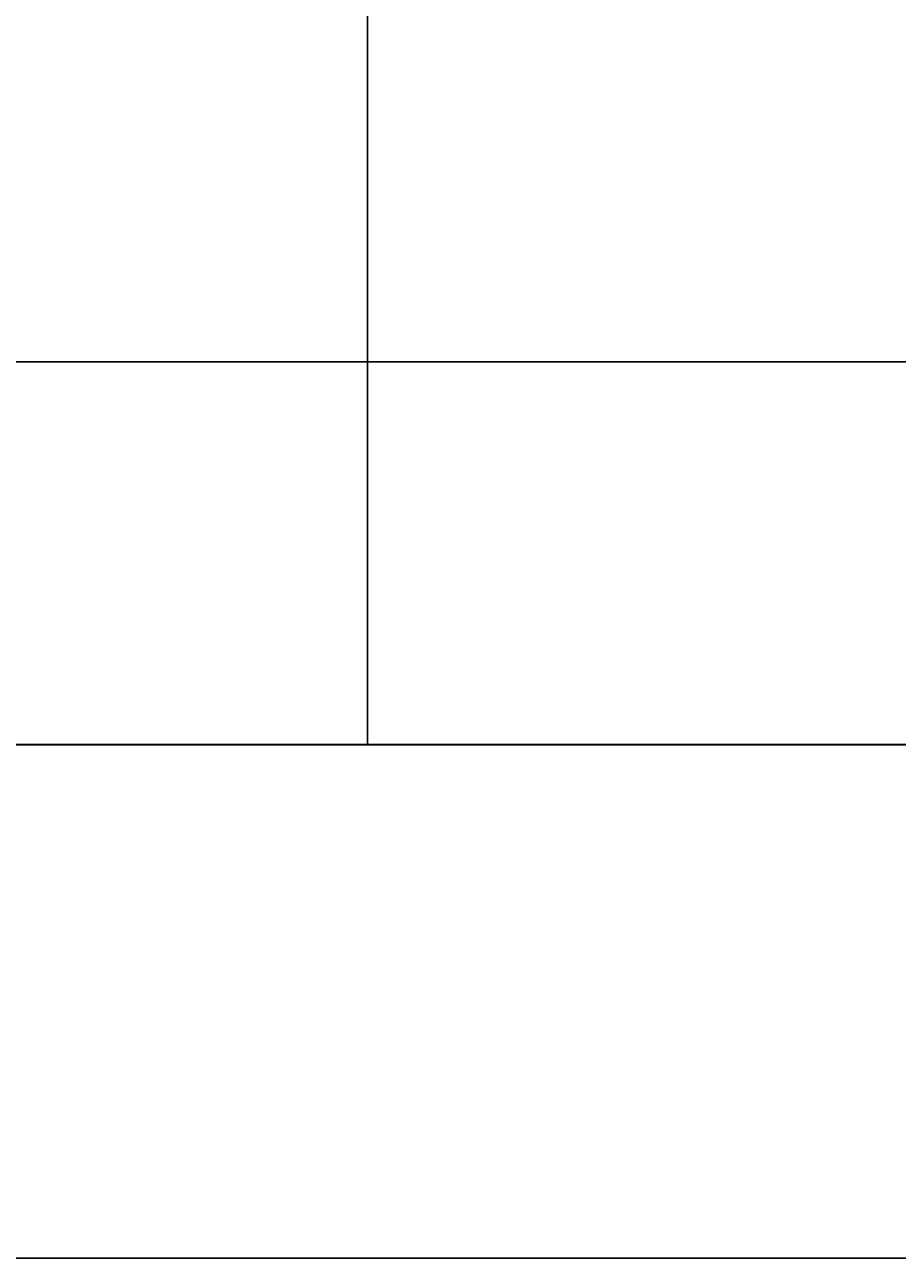
# Model space of a CAD drawing. Units: inches. Extents: x -26 to 776, y -22 to 650.
# Tile 2 of 62: x 36 to 98, y -22 to 67. Entities that reach past the tile are written whole.
import ezdxf

# ---------------------------------------------------------------- set-up
doc = ezdxf.new("R2010")
doc.units = ezdxf.units.IN
doc.header["$MEASUREMENT"] = 0
for name, color, linetype, lineweight in [('A-ANNO-DIMS', 2, 'Continuous', 18), ('A-DOOR', 3, 'Continuous', 25), ('C-TOPO', 7, 'Continuous', 35)]:
    doc.layers.add(name, color=color, linetype=linetype, lineweight=lineweight)
doc.styles.get("Standard").update_dxf_attribs({"font": 'arial.ttf'})
doc.dimstyles.get("Standard").update_dxf_attribs({"dimtxt": 0.5625, "dimasz": 0.18, "dimexe": 0.18, "dimexo": 0.0625, "dimgap": 0.09, "dimtad": 0, "dimtih": 1, "dimtoh": 1, "dimdec": 4, "dimzin": 0, "dimdsep": 46, "dimlunit": 4, "dimtxsty": 'Standard', "dimcen": 0.09, "dimadec": 0, "dimazin": 0, "dimtfac": 1, "dimtdec": 4, "dimtofl": 0, "dimtmove": 0, "dimatfit": 3, "dimfxl": 1, "dimtolj": 1, "dimtzin": 0, "dimarcsym": 0})

# ---------------------------------------------------------------- blocks, each defined once
blk = doc.blocks.new('*D13')
at = {"layer": 'A-ANNO-DIMS', "color": 0, "lineweight": -2, "transparency": 16777216}
for p, q in [((738.75, 50.786), (738.75, -21.315)), ((11.107, 15.42), (11.107, -21.315)), ((11.287, -21.135), (373.892, -21.135)), ((738.57, -21.135), (375.965, -21.135))]:
    blk.add_line(p, q, dxfattribs=at)
at = {"layer": 'A-ANNO-DIMS', "color": 0, "transparency": 16777216}
for points in [[(11.287, -21.105), (11.287, -21.165), (11.107, -21.135)], [(738.57, -21.105), (738.57, -21.165), (738.75, -21.135)]]:
    blk.add_solid(points, dxfattribs=at)
at = {"layer": 'Defpoints', "color": 0, "transparency": 16777216}
for p in [(738.75, 50.848), (11.107, 15.482), (738.75, -21.135)]:
    blk.add_point(p, dxfattribs=at)
at = {"layer": 'A-ANNO-DIMS', "color": 0, "transparency": 16777216, "insert": (374.929, -21.135), "char_height": 0.5625, "attachment_point": 5}
blk.add_mtext('\\A1;727.6', dxfattribs=at)
blk = doc.blocks.new('*D14')
at = {"layer": 'A-ANNO-DIMS', "color": 0, "lineweight": -2, "transparency": 16777216}
for p, q in [((191.616, 613.271), (-25.478, 613.271)), ((-25.298, 613.091), (-25.298, 314.754)), ((-25.298, 15.662), (-25.298, 314)), ((11.045, 15.482), (-25.478, 15.482))]:
    blk.add_line(p, q, dxfattribs=at)
at = {"layer": 'A-ANNO-DIMS', "color": 0, "transparency": 16777216}
for points in [[(-25.328, 613.091), (-25.268, 613.091), (-25.298, 613.271)], [(-25.328, 15.662), (-25.268, 15.662), (-25.298, 15.482)]]:
    blk.add_solid(points, dxfattribs=at)
at = {"layer": 'Defpoints', "color": 0, "transparency": 16777216}
for p in [(-25.298, 613.271), (191.678, 613.271), (11.107, 15.482)]:
    blk.add_point(p, dxfattribs=at)
at = {"layer": 'A-ANNO-DIMS', "color": 0, "transparency": 16777216, "insert": (-25.298, 314.377), "char_height": 0.5625, "attachment_point": 5}
blk.add_mtext('\\A1;597.8', dxfattribs=at)
blk = doc.blocks.new('*D22')
at = {"layer": 'A-ANNO-DIMS', "color": 0, "lineweight": -2, "transparency": 16777216}
for p, q in [((22.889, 15.333), (22.889, 649.856)), ((217.953, 15.545), (217.953, 649.856)), ((23.069, 649.676), (119.19, 649.676)), ((217.773, 649.676), (121.652, 649.676))]:
    blk.add_line(p, q, dxfattribs=at)
at = {"layer": 'A-ANNO-DIMS', "color": 0, "transparency": 16777216}
for points in [[(23.069, 649.706), (23.069, 649.646), (22.889, 649.676)], [(217.773, 649.706), (217.773, 649.646), (217.953, 649.676)]]:
    blk.add_solid(points, dxfattribs=at)
at = {"layer": 'Defpoints', "color": 0, "transparency": 16777216}
for p in [(217.953, 649.676), (22.889, 15.27), (217.953, 15.482)]:
    blk.add_point(p, dxfattribs=at)
at = {"layer": 'A-ANNO-DIMS', "color": 0, "transparency": 16777216, "insert": (120.421, 649.676), "char_height": 0.5625, "attachment_point": 5}
blk.add_mtext('\\A1;195.06', dxfattribs=at)
blk = doc.blocks.new('*D37')
at = {"layer": 'A-ANNO-DIMS', "color": 0, "lineweight": -2, "transparency": 16777216}
for p, q in [((231.362, 159.482), (-25.478, 159.482)), ((-25.298, 159.302), (-25.298, 87.855)), ((-25.298, 15.662), (-25.298, 87.11)), ((217.89, 15.482), (-25.478, 15.482))]:
    blk.add_line(p, q, dxfattribs=at)
at = {"layer": 'A-ANNO-DIMS', "color": 0, "transparency": 16777216}
for points in [[(-25.328, 159.302), (-25.268, 159.302), (-25.298, 159.482)], [(-25.328, 15.662), (-25.268, 15.662), (-25.298, 15.482)]]:
    blk.add_solid(points, dxfattribs=at)
at = {"layer": 'Defpoints', "color": 0, "transparency": 16777216}
for p in [(-25.298, 159.482), (231.425, 159.482), (217.953, 15.482)]:
    blk.add_point(p, dxfattribs=at)
at = {"layer": 'A-ANNO-DIMS', "color": 0, "transparency": 16777216, "insert": (-25.298, 87.482), "char_height": 0.5625, "attachment_point": 5}
blk.add_mtext('\\A1;144', dxfattribs=at)

msp = doc.modelspace()

# ---------------------------------------------------------------- linework, layer by layer
at = {"layer": 'A-DOOR'}
for p, q in [((60.2178, 124.9232), (60.2178, 15.4824)), ((22.8891, 42.7535), (217.9529, 42.7535))]:
    msp.add_line(p, q, dxfattribs=at)
at = {"layer": 'C-TOPO'}
for p, q in [((11.1074, 15.4824), (92.2983, 15.4824)), ((92.2983, 15.4824), (214.0443, 15.4824))]:
    msp.add_line(p, q, dxfattribs=at)

# ---------------------------------------------------------------- dimensions: what is measured, and where the dimension line sits
at = {"layer": 'A-ANNO-DIMS'}
for base, p1, p2, override, picture, middle in [((217.9529, 649.6763), (22.8891, 15.2701), (217.9529, 15.4824), {"dimdec": 2, "dimlfac": 1, "dimrnd": 0, "dimzin": 0, "dimdsep": 46, "dimlunit": 2}, '*D22', (120.421, 649.6763)), ((738.7503, -21.1349), (11.1074, 15.4824), (738.7503, 50.8482), {"dimdec": 1, "dimlfac": 1, "dimrnd": 0, "dimzin": 0, "dimdsep": 46, "dimlunit": 2}, '*D13', (374.9289, -21.1349))]:
    dim = msp.add_linear_dim(base=base, p1=p1, p2=p2, dimstyle='Standard', override=override, dxfattribs=at)
    dim.commit()
    dim.dimension.update_dxf_attribs({"geometry": picture, "text_midpoint": middle})
for base, p1, p2, override, picture, middle in [((-25.2976, 613.2713), (11.1074, 15.4824), (191.6782, 613.2713), {"dimdec": 1, "dimlfac": 1, "dimrnd": 0, "dimzin": 0, "dimdsep": 46, "dimlunit": 2}, '*D14', (-25.2976, 314.3769)), ((-25.2976, 159.4824), (217.9529, 15.4824), (231.4249, 159.4824), {"dimdec": 0, "dimlfac": 1, "dimrnd": 0, "dimzin": 0, "dimdsep": 46, "dimlunit": 2}, '*D37', (-25.2976, 87.4824))]:
    dim = msp.add_linear_dim(base=base, p1=p1, p2=p2, angle=90, dimstyle='Standard', override=override, dxfattribs=at)
    dim.commit()
    dim.dimension.update_dxf_attribs({"geometry": picture, "text_midpoint": middle})

doc.saveas('drawing.dxf')
